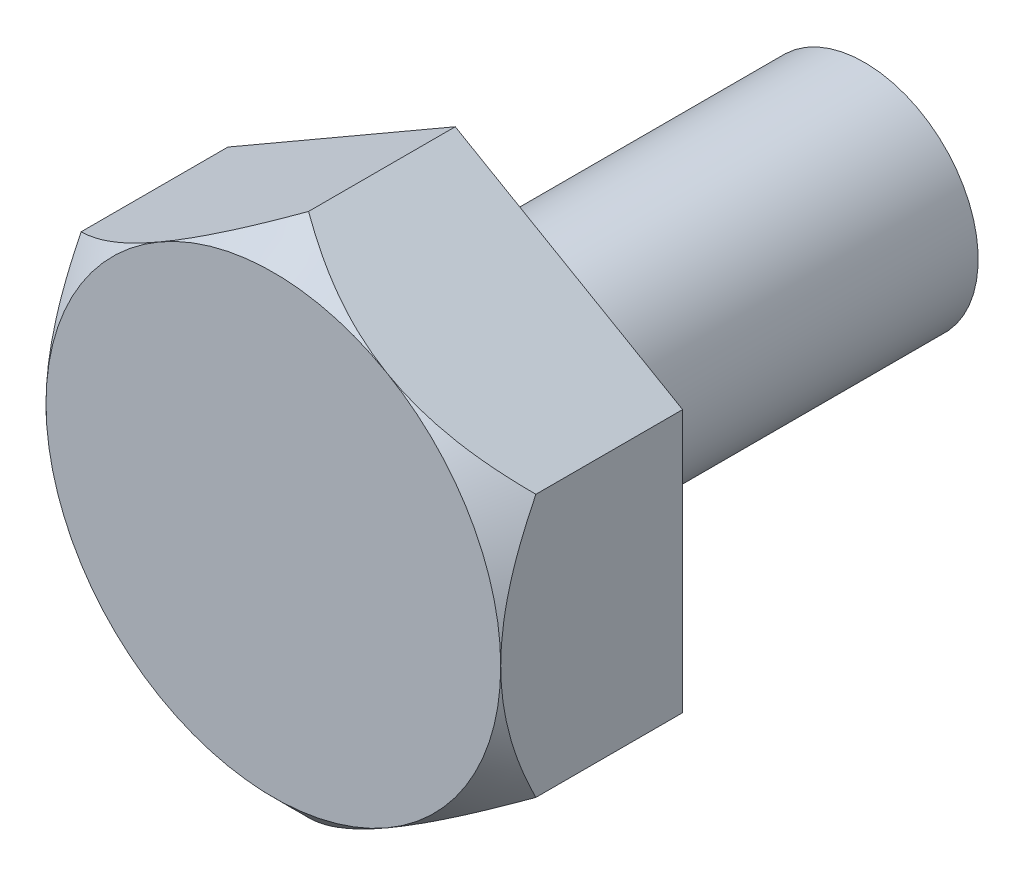
from build123d import *

# Parameters (mm, degrees)
HEX_HEAD_DEPTH                 = 4
HEAD_CHAMFER_PROFILE_OUTSIDE_W = 23.158
HEAD_CHAMFER_PROFILE_OUTSIDE_H = 24.706
HEAD_CHAMFER_PROFILE_OUTSIDE_R = 5
HEAD_CHAMFER_45DEG_DEPTH       = 4
HEAD_CHAMFER_45DEG_DRAFT       = -45
SHANK_PROFILE_5_R              = 2.5
SHANK_5X9_DEPTH                = 9


with BuildPart() as part:
    # Hex Head Profile → Hex Head (new body)
    with BuildSketch(Plane.XY):
        Polygon((5, -2.886751346), (5, 2.886751346), (0, 5.773502692), (-5, 2.886751346), (-5, -2.886751346), (0, -5.773502692), align=None)
    extrude(amount=HEX_HEAD_DEPTH)


with BuildPart() as head_chamfer_45deg_tool:
    # Head Chamfer Profile outside → Head Chamfer 45deg (with draft: the straight prism first)
    with BuildSketch(Plane.XY.offset(4)):
        Rectangle(HEAD_CHAMFER_PROFILE_OUTSIDE_W, HEAD_CHAMFER_PROFILE_OUTSIDE_H)
        Circle(HEAD_CHAMFER_PROFILE_OUTSIDE_R, mode=Mode.SUBTRACT)
    extrude(amount=-HEAD_CHAMFER_45DEG_DEPTH)
    # Head Chamfer 45deg: the draft: its side faces are tilted about the plane it starts from
    head_chamfer_45deg_sides = [head_chamfer_45deg_tool.faces().sort_by_distance(p)[0] for p in [
        (0, -12.353, 2),
        (11.579, 0, 2),
        (0, 12.353, 2),
        (-11.579, 0, 2),
        (-5, 0, 2),
    ]]
    draft(head_chamfer_45deg_sides, Plane.XY.offset(4), HEAD_CHAMFER_45DEG_DRAFT)


with BuildPart() as part_1:
    add(part.part)

    # Head Chamfer 45deg: cut by head_chamfer_45deg_tool
    add(head_chamfer_45deg_tool.part, mode=Mode.SUBTRACT)

    # Shank Profile Ø5 → Shank Ø5x9 (add)
    with BuildSketch(Plane(origin=(0, 0, 0), x_dir=(-1, 0, 0), z_dir=(0, 0, -1))):
        Circle(SHANK_PROFILE_5_R)
    extrude(amount=SHANK_5X9_DEPTH)


solid = part_1.part
